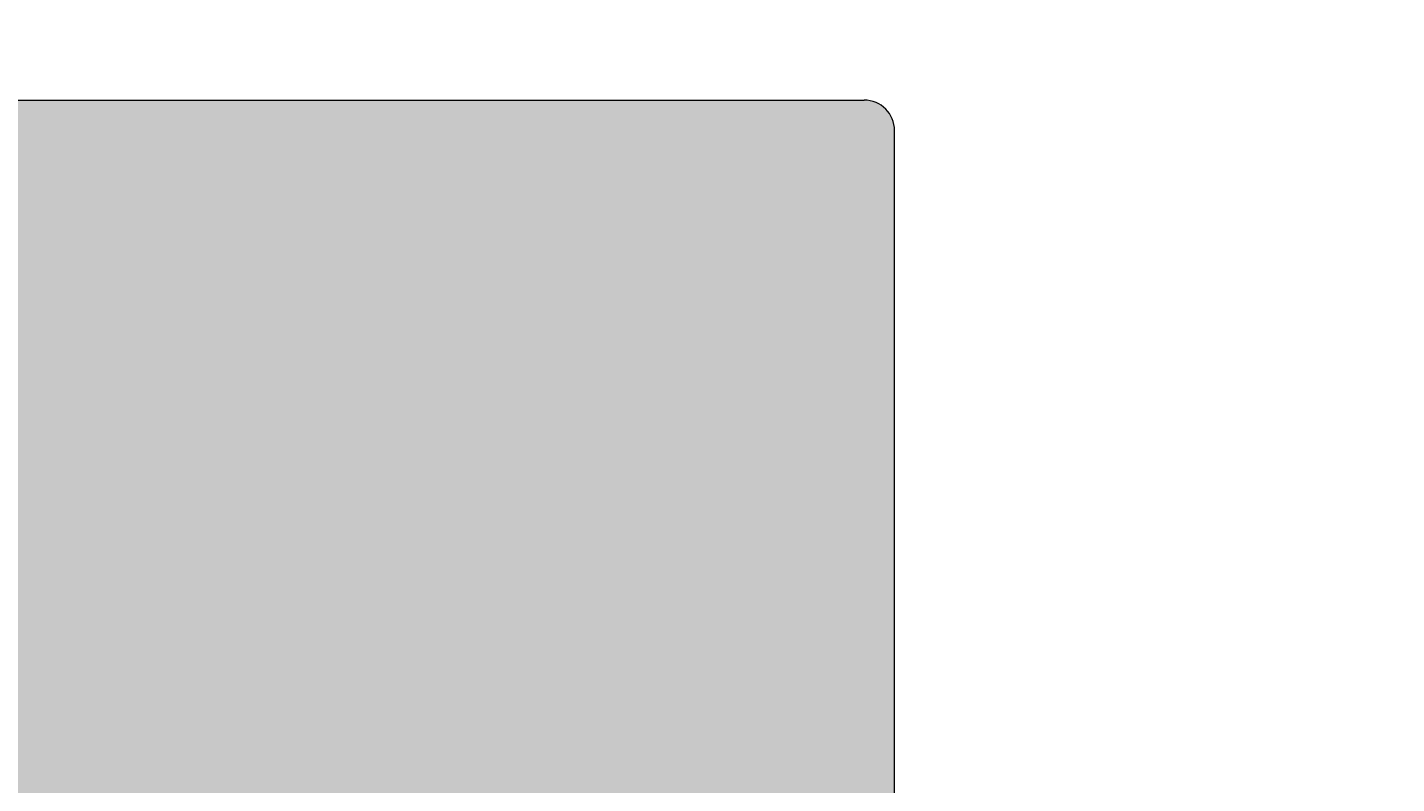
# Model space of a CAD drawing. Units: millimetres. Extents: x 27017497 to 27018854, y 7058029 to 7059154.
# Tile 77 of 91: x 27018390 to 27018462, y 7058185 to 7058224. Entities that reach past the tile are written whole.
import ezdxf

# ---------------------------------------------------------------- set-up
doc = ezdxf.new("R2010")
doc.units = ezdxf.units.MM
doc.layers.add('A-ANNO-DIMS', color=2, linetype='Continuous', lineweight=18)
doc.layers.add('A-FURN', color=8, linetype='Continuous', lineweight=18)
doc.layers.add('A-FURN-PATT', color=177, linetype='Continuous', lineweight=13, true_color=0x293189)
doc.styles.get("Standard").update_dxf_attribs({"font": 'arial.ttf'})
doc.dimstyles.get("Standard").update_dxf_attribs({"dimtxt": 0.18, "dimasz": 0.18, "dimexe": 0.18, "dimexo": 0.0625, "dimgap": 0.09, "dimtad": 0, "dimtih": 1, "dimtoh": 1, "dimdec": 4, "dimzin": 0, "dimdsep": 46, "dimtxsty": 'Standard', "dimcen": 0.09, "dimadec": 0, "dimazin": 0, "dimtfac": 1, "dimtdec": 4, "dimtofl": 0, "dimtmove": 0, "dimatfit": 3, "dimfxl": 1, "dimtolj": 1, "dimtzin": 0, "dimarcsym": 0})

# ---------------------------------------------------------------- blocks, each defined once
blk = doc.blocks.new('CAMMAT')
for p, q in [((-0.65, -0.8139), (-0.65, -1.93)), ((0.61, -1.97), (-0.61, -1.97))]:
    blk.add_line(p, q)
blk.add_arc((-0.61, -1.93), 0.04, 180, 270)
blk = doc.blocks.new('*D47')
at = {"layer": 'A-ANNO-DIMS', "color": 0, "lineweight": -2, "transparency": 16777216}
for p, q in [((27017561.166, 7058294.35), (27017561.166, 7058028.6)), ((27018790.606, 7058294.35), (27018790.606, 7058028.6)), ((27017561.346, 7058028.78), (27018175.431, 7058028.78)), ((27018790.426, 7058028.78), (27018176.341, 7058028.78))]:
    blk.add_line(p, q, dxfattribs=at)
at = {"layer": 'A-ANNO-DIMS', "color": 0, "transparency": 16777216}
for points in [[(27017561.346, 7058028.81), (27017561.346, 7058028.75), (27017561.166, 7058028.78)], [(27018790.426, 7058028.81), (27018790.426, 7058028.75), (27018790.606, 7058028.78)]]:
    blk.add_solid(points, dxfattribs=at)
at = {"layer": 'Defpoints', "color": 0, "transparency": 16777216}
for p in [(27017561.166, 7058294.412), (27018790.606, 7058294.412), (27018790.606, 7058028.78)]:
    blk.add_point(p, dxfattribs=at)
at = {"layer": 'A-ANNO-DIMS', "color": 0, "transparency": 16777216, "insert": (27018175.886, 7058028.78), "char_height": 0.18, "attachment_point": 5}
blk.add_mtext('\\A1;1229.4', dxfattribs=at)
blk = doc.blocks.new('*D48')
at = {"layer": 'A-ANNO-DIMS', "color": 0, "lineweight": -2, "transparency": 16777216}
for p, q in [((27018463.498, 7058622.912), (27017497.536, 7058622.912)), ((27017497.716, 7058622.732), (27017497.716, 7058357.753)), ((27017497.716, 7058092.41), (27017497.716, 7058357.389)), ((27018555.129, 7058092.23), (27017497.536, 7058092.23))]:
    blk.add_line(p, q, dxfattribs=at)
at = {"layer": 'A-ANNO-DIMS', "color": 0, "transparency": 16777216}
for points in [[(27017497.686, 7058622.732), (27017497.746, 7058622.732), (27017497.716, 7058622.912)], [(27017497.686, 7058092.41), (27017497.746, 7058092.41), (27017497.716, 7058092.23)]]:
    blk.add_solid(points, dxfattribs=at)
at = {"layer": 'Defpoints', "color": 0, "transparency": 16777216}
for p in [(27018463.561, 7058622.912), (27017497.716, 7058092.23), (27018555.192, 7058092.23)]:
    blk.add_point(p, dxfattribs=at)
at = {"layer": 'A-ANNO-DIMS', "color": 0, "transparency": 16777216, "insert": (27017497.716, 7058357.571), "char_height": 0.18, "attachment_point": 5}
blk.add_mtext('\\A1;530.7', dxfattribs=at)

msp = doc.modelspace()

# ---------------------------------------------------------------- hatches: boundary and pattern name
at = {"layer": 'A-FURN-PATT'}
h = msp.add_hatch(color=256, dxfattribs=at)
h.dxf.hatch_style = 1
h.paths.add_polyline_path([(27018435.86, 7058218.784, 0.414214), (27018434.267, 7058220.377), (27018385.674, 7058220.377, 0.414214), (27018384.081, 7058218.784), (27018384.081, 7058174.59), (27018387.977, 7058174.891), (27018391.56, 7058175.393), (27018394.078, 7058176.128), (27018395.791, 7058177.21), (27018396.958, 7058178.748), (27018397.838, 7058180.854), (27018398.69, 7058183.639), (27018399.293, 7058180.835), (27018399.836, 7058178.594), (27018400.426, 7058176.691), (27018401.17, 7058174.899), (27018402.177, 7058172.991), (27018403.552, 7058170.741), (27018405.403, 7058167.922), (27018407.838, 7058164.308), (27018410.273, 7058167.922), (27018412.124, 7058170.741), (27018413.499, 7058172.991), (27018414.506, 7058174.899), (27018415.25, 7058176.691), (27018415.84, 7058178.594), (27018416.383, 7058180.835), (27018416.986, 7058183.639), (27018417.838, 7058180.854), (27018418.718, 7058178.748), (27018419.885, 7058177.21), (27018421.598, 7058176.128), (27018424.116, 7058175.393), (27018427.699, 7058174.891), (27018432.604, 7058174.513), (27018435.86, 7058174.329)])
h.paths.add_polyline_path([(27018439.093, 7058174.146), (27018432.604, 7058174.513), (27018427.699, 7058174.891), (27018424.116, 7058175.393), (27018421.598, 7058176.128), (27018419.885, 7058177.21), (27018418.718, 7058178.748), (27018417.838, 7058180.854), (27018416.986, 7058183.639), (27018416.383, 7058180.835), (27018415.84, 7058178.594), (27018415.25, 7058176.691), (27018414.506, 7058174.899), (27018413.499, 7058172.991), (27018412.124, 7058170.741), (27018410.273, 7058167.922), (27018407.838, 7058164.308)])
h.paths.add_polyline_path([(27018403.552, 7058170.741), (27018402.177, 7058172.991), (27018401.17, 7058174.899), (27018400.426, 7058176.691), (27018399.836, 7058178.594), (27018399.293, 7058180.835), (27018398.69, 7058183.639), (27018397.838, 7058180.854), (27018396.958, 7058178.748), (27018395.791, 7058177.21), (27018394.078, 7058176.128), (27018391.56, 7058175.393), (27018387.977, 7058174.891), (27018383.071, 7058174.513), (27018376.583, 7058174.146), (27018407.838, 7058164.308), (27018405.403, 7058167.922)])
h.paths.add_polyline_path([(27018437.469, 7058173.635), (27018407.838, 7058164.308), (27018382.784, 7058172.194), (27018382.784, 7058162.502), (27018437.469, 7058162.502)])
h.paths.add_polyline_path([(27018435.86, 7058162.502), (27018384.081, 7058162.502), (27018384.081, 7058146.294, 0.414214), (27018385.674, 7058144.7), (27018434.267, 7058144.7, 0.414214), (27018435.86, 7058146.294)])
h.paths.add_polyline_path([(27018407.684, 7058159.418, -0.41419), (27018408.879, 7058158.223), (27018408.879, 7058148.664, -0.414237), (27018407.684, 7058147.469), (27018386.224, 7058147.469, -0.41419), (27018385.029, 7058148.663), (27018385.029, 7058158.223, -0.414237), (27018386.224, 7058159.418)], flags=16)
h.paths.add_polyline_path([(27018411.821, 7058159.418), (27018433.28, 7058159.418, -0.41419), (27018434.475, 7058158.223), (27018434.475, 7058148.664, -0.414237), (27018433.28, 7058147.469), (27018411.821, 7058147.469, -0.414214), (27018410.626, 7058148.664), (27018410.626, 7058158.223, -0.414214)], flags=16)
h.paths.add_polyline_path([(27018382.886, 7058160.632), (27018362.971, 7058160.632), (27018362.971, 7058144.7), (27018382.886, 7058144.7)])
h.paths.add_polyline_path([(27018379.136, 7058152.033, -1), (27018367.187, 7058152.033, -1)], flags=16)
h.paths.add_polyline_path([(27018376.861, 7058152.033, -1), (27018369.461, 7058152.033, -1)], flags=0)
h.paths.add_polyline_path([(27018456.97, 7058160.632), (27018437.055, 7058160.632), (27018437.055, 7058144.7), (27018456.97, 7058144.7)])
h.paths.add_polyline_path([(27018453.028, 7058152.033, -1), (27018441.079, 7058152.033, -1)], flags=16)
h.paths.add_polyline_path([(27018450.754, 7058152.033, -1), (27018443.354, 7058152.033, -1)], flags=0)
h.paths.add_polyline_path([(27018434.475, 7058158.223, 0.41419), (27018433.28, 7058159.418), (27018411.821, 7058159.418, 0.414214), (27018410.626, 7058158.223), (27018410.626, 7058148.664, 0.414214), (27018411.821, 7058147.469), (27018433.28, 7058147.469, 0.414237), (27018434.475, 7058148.664)], flags=0)

# ---------------------------------------------------------------- block references
at = {"layer": 'A-FURN', "xscale": 39.82996475819422, "yscale": 39.82996475819422, "zscale": 39.82996475819422, "rotation": 180}
msp.add_blockref('CAMMAT', (27018409.97, 7058141.912), dxfattribs=at)

# ---------------------------------------------------------------- dimensions: what is measured, and where the dimension line sits
at = {"layer": 'A-ANNO-DIMS'}
dim = msp.add_linear_dim(base=(27017497.716, 7058092.23), p1=(27018463.561, 7058622.912), p2=(27018555.192, 7058092.23), angle=90, dimstyle='Standard', override={"dimdec": 1, "dimlfac": 1, "dimrnd": 0, "dimzin": 0, "dimdsep": 46, "dimlunit": 2}, dxfattribs=at)
dim.commit()
dim.dimension.update_dxf_attribs({"geometry": '*D48', "text_midpoint": (27017497.716, 7058357.571)})
dim = msp.add_linear_dim(base=(27018790.606, 7058028.78), p1=(27017561.166, 7058294.412), p2=(27018790.606, 7058294.412), dimstyle='Standard', override={"dimdec": 1, "dimlfac": 1, "dimrnd": 0, "dimzin": 0, "dimdsep": 46, "dimlunit": 2}, dxfattribs=at)
dim.commit()
dim.dimension.update_dxf_attribs({"geometry": '*D47', "text_midpoint": (27018175.886, 7058028.78)})

doc.saveas('drawing.dxf')
